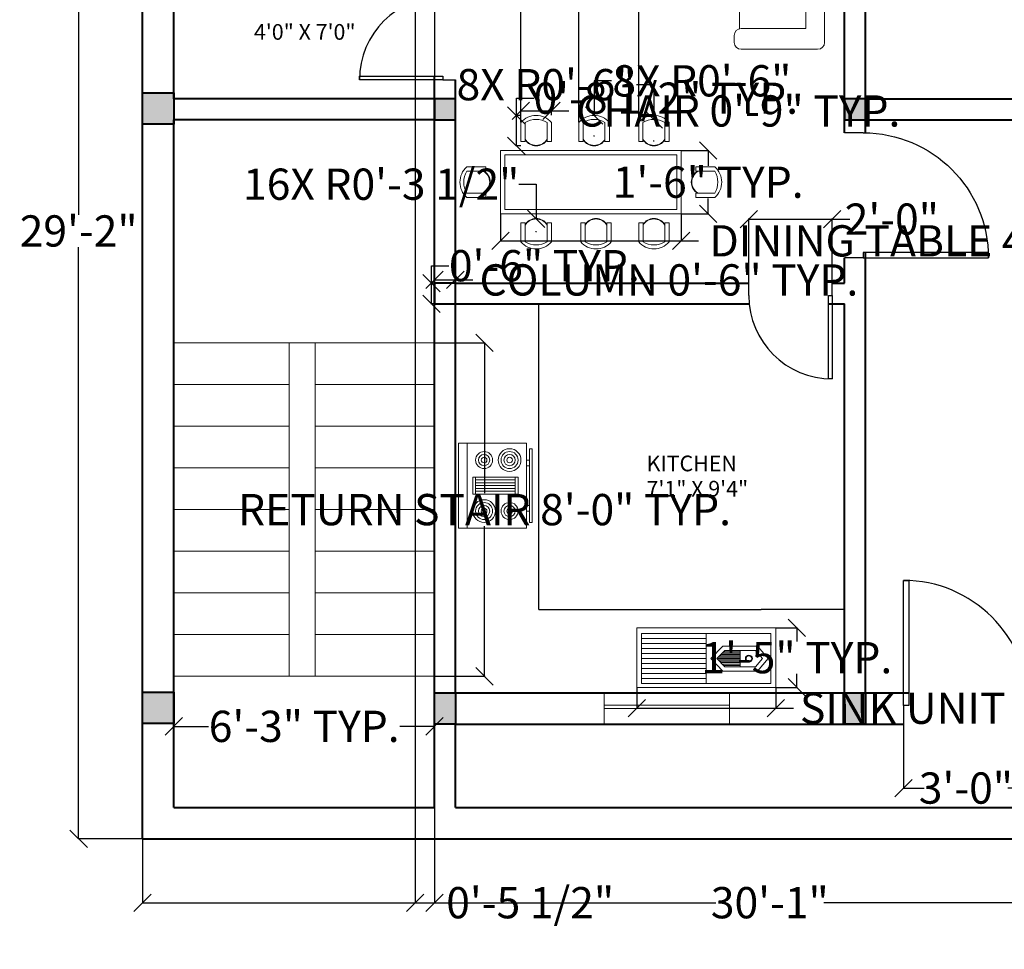
# Model space of a CAD drawing. Units: inches. Extents: x -19 to 1000, y -122 to 1144.
# Tile 1 of 8: x -14 to 270, y -122 to 146. Entities that reach past the tile are written whole.
import ezdxf

# ---------------------------------------------------------------- set-up
doc = ezdxf.new("R2010")
doc.units = ezdxf.units.IN
doc.header["$MEASUREMENT"] = 0
for name, color, linetype, lineweight in [('A-ANNO-DIMS', 191, 'Continuous', 18), ('A-AREA-IDEN', 1, 'Continuous', 18), ('A-COLS', 4, 'Continuous', 40), ('A-COLS-PATT', 220, 'Continuous', 13), ('A-EQPM', 120, 'Continuous', 18), ('A-FLOR-CASE', 254, 'Continuous', 25), ('A-FLOR-FIXT', 8, 'Continuous', 18), ('A-FLOR-STRS', 241, 'Continuous', 18), ('DOORS', 2, 'Continuous', 25), ('FURNITURE', 120, 'Continuous', 18), ('WALLS', 4, 'Continuous', 40), ('WINDOWS', 3, 'Continuous', 18)]:
    doc.layers.add(name, color=color, linetype=linetype, lineweight=lineweight)
doc.styles.get("Standard").update_dxf_attribs({"font": 'arial.ttf'})
doc.dimstyles.get("Standard").update_dxf_attribs({"dimtxt": 9, "dimasz": 5, "dimexe": 0.18, "dimexo": 0.0625, "dimgap": 0.09, "dimtad": 0, "dimtih": 1, "dimtoh": 1, "dimdec": 0, "dimzin": 0, "dimdsep": 46, "dimlunit": 3, "dimtxsty": 'Standard', "dimblk": 'OBLIQUE', "dimcen": 0.09, "dimadec": 0, "dimazin": 0, "dimtfac": 1, "dimtdec": 0, "dimtofl": 0, "dimtmove": 0, "dimatfit": 3, "dimfxl": 1, "dimtolj": 1, "dimtzin": 0, "dimarcsym": 0})

# ---------------------------------------------------------------- blocks, each defined once
blk = doc.blocks.new('Range-Oven - 30 in top')
for p, q in [((0, -3), (30, -3)), ((12, -6), (18, -6)), ((13, -20), (13, -6)), ((14, -6), (14, -20)), ((15, -20), (15, -6)), ((16, -6), (16, -20)), ((17, -20), (17, -6)), ((18, -20), (12, -20)), ((6, -24), (6, -25)), ((8, -25), (8, -24)), ((22, -25), (22, -24)), ((24, -24), (24, -25))]:
    blk.add_line(p, q)
for points in [[(0, -24), (0, 0), (30, 0), (30, -24)], [(12, -21), (12, -5), (18, -5), (18, -21)], [(2, -26), (2, -25), (28, -25), (28, -26)]]:
    blk.add_lwpolyline(points, close=True)
for centre, radius in [((6, -9), 4), ((6, -9), 3), ((24, -9), 3), ((6, -9), 2), ((6, -9), 1), ((24, -9), 2), ((24, -9), 1), ((6, -18), 3), ((6, -18), 2), ((6, -18), 1), ((24, -18), 4), ((24, -18), 3), ((24, -18), 2), ((24, -18), 1)]:
    blk.add_circle(centre, radius)
blk = doc.blocks.new('*U3')
for p, q in [((0, 0), (0, -6)), ((40, 0), (40, -6))]:
    blk.add_line(p, q)
blk.add_lwpolyline([(0, 0), (0, 40), (1.75, 40), (1.75, 0)], close=True)
blk.add_arc((0, 0), 40, 0, 90)
blk = doc.blocks.new('SOFA-THREE-SEAT')
for p, q in [((2, 84), (24, 84)), ((0, 78), (0, 82)), ((26, 82), (26, 2)), ((0, 78), (20.62, 78)), ((1.56, 78), (1.56, 56)), ((20.62, 78), (20.62, 6)), ((3.56, 54), (20.62, 54)), ((3.56, 54), (3.56, 54)), ((1.56, 52), (1.56, 32)), ((3.56, 30), (20.62, 30)), ((3.56, 30), (3.56, 30)), ((1.56, 28), (1.56, 6)), ((2, 6), (20.62, 6)), ((0, 2), (0, 4)), ((24, 0), (2, 0))]:
    blk.add_line(p, q)
for centre, start, end in [((2, 82), 90, 180), ((24, 82), 0, 90), ((3.56, 56), 180, 270), ((3.56, 52), 90, 180), ((3.56, 32), 180, 270), ((3.56, 28), 90, 180), ((2, 4), 90, 180), ((2, 2), 180, 270), ((24, 2), 270, 0)]:
    blk.add_arc(centre, 2, start, end)
blk = doc.blocks.new('TABLE-DINING')
for points in [[(51.97, 0), (0, 0), (0, 18.2), (51.97, 18.2)], [(50.72, 1.24), (1.24, 1.24), (1.24, 16.96), (50.72, 16.96)]]:
    blk.add_lwpolyline(points, close=True)
blk = doc.blocks.new('CHAIR-DINING')
for p, q in [((0, 1.28), (0, 6.78)), ((1.24, 1.28), (1.24, 6.78)), ((7.52, 1.28), (7.52, 6.78)), ((8.77, 1.28), (8.77, 6.78)), ((0, 1.28), (1.24, 1.28)), ((7.52, 1.28), (8.77, 1.28))]:
    blk.add_line(p, q)
for centre, radius, start, end in [((4.38, 2.88), 5.87, 41.6504, 138.3496), ((4.38, 1.47), 6.17, 59.4137, 120.5863), ((4.38, 3.81), 3.65, 210.7965, 329.2035), ((4.38, 3.65), 3.65, 210.7965, 329.2035)]:
    blk.add_arc(centre, radius, start, end)
blk = doc.blocks.new('SINK-WITH-DRAINBOARD')
for p, q in [((19.91, 15.5), (1.26, 15.5)), ((19.91, 1.08), (19.91, 15.5)), ((19.91, 14.06), (1.26, 14.06)), ((19.91, 12.62), (1.26, 12.62)), ((24.75, 11.88), (21.21, 8.28)), ((24.75, 11.88), (34.73, 11.88)), ((34.73, 11.88), (37.76, 8.28)), ((19.91, 11.17), (1.26, 11.17)), ((19.91, 9.73), (1.26, 9.73)), ((25.28, 10.62), (22.97, 8.28)), ((23.36, 8.67), (29.71, 8.67)), ((23.74, 9.06), (29.71, 9.06)), ((24.12, 9.45), (29.71, 9.45)), ((24.51, 9.84), (29.71, 9.84)), ((24.89, 10.23), (29.71, 10.23)), ((25.28, 10.62), (34.14, 10.62)), ((25.28, 10.62), (29.71, 10.62)), ((29.71, 5.94), (29.71, 10.62)), ((34.14, 10.62), (36.12, 8.28)), ((19.91, 8.29), (1.26, 8.29)), ((19.91, 6.85), (1.26, 6.85)), ((24.75, 4.68), (21.21, 8.28)), ((25.28, 5.94), (22.97, 8.28)), ((22.97, 8.28), (29.71, 8.28)), ((23.36, 7.89), (29.71, 7.89)), ((23.74, 7.5), (29.71, 7.5)), ((24.12, 7.11), (29.71, 7.11)), ((24.51, 6.72), (29.71, 6.72)), ((24.89, 6.33), (29.71, 6.33)), ((25.28, 5.94), (34.14, 5.94)), ((34.14, 5.94), (36.12, 8.28)), ((34.73, 4.68), (37.76, 8.28)), ((19.91, 5.4), (1.26, 5.4)), ((19.91, 3.96), (1.26, 3.96)), ((24.75, 4.68), (34.73, 4.68)), ((19.91, 2.52), (1.26, 2.52))]:
    blk.add_line(p, q)
for points in [[(40, 0), (0, 0), (0, 17.1), (40, 17.1)], [(38.55, 1.08), (1.26, 1.08), (1.26, 15.5), (38.55, 15.5)]]:
    blk.add_lwpolyline(points, close=True)
for radius in [1.01, 0.803]:
    blk.add_circle((32.21, 8.28), radius)
blk = doc.blocks.new('STAIR-RETURN-PLAN')
for p, q in [((75, 96), (0, 96)), ((33.21, 0), (33.21, 96)), ((40.68, 0), (40.68, 96)), ((33.21, 84), (0, 84)), ((75, 84), (40.68, 84)), ((33.21, 72), (0, 72)), ((75, 72), (40.68, 72)), ((33.21, 60), (0, 60)), ((75, 60), (40.68, 60)), ((33.21, 48), (0, 48)), ((75, 48), (40.68, 48)), ((33.21, 36), (0, 36)), ((75, 36), (40.68, 36)), ((33.21, 24), (0, 24)), ((75, 24), (40.68, 24)), ((33.21, 12), (0, 12)), ((75, 12), (40.68, 12)), ((75, 0), (0, 0))]:
    blk.add_line(p, q)
blk = doc.blocks.new('WIN-36-PLAN')
for p, q in [((0, 4.5), (0, 9)), ((0, 9), (0, 0)), ((36, 9), (36, 0)), ((0, 5.5), (36, 5.5)), ((0, 5.5), (36, 5.5)), ((0, 4.5), (36, 4.5))]:
    blk.add_line(p, q)
blk = doc.blocks.new('COLUMN-9X9')
blk.add_lwpolyline([(0, 9), (9, 9), (9, 0), (0, 0)], close=True)
blk = doc.blocks.new('COLUMN-6X6')
blk.add_lwpolyline([(6, 6), (0, 6), (0, 0), (6, 0)], close=True)
blk = doc.blocks.new('COLUMN-6X9')
blk.add_lwpolyline([(0, 9), (6, 9), (6, 0), (0, 0)], close=True)
blk = doc.blocks.new('_Oblique')
at = {"color": 0, "linetype": 'ByBlock', "lineweight": -2}
blk.add_line((-0.5, -0.5), (0.5, 0.5), dxfattribs=at)
blk = doc.blocks.new('*D35')
at = {"layer": 'A-ANNO-DIMS', "color": 0, "lineweight": -2, "transparency": 16777216}
for p, q in [((105.64, 69.78), (105.64, 70.79)), ((105.64, 70.61), (111.64, 70.61)), ((111.64, 69.78), (111.64, 70.79)), ((111.64, 70.61), (116.64, 70.61))]:
    blk.add_line(p, q, dxfattribs=at)
at = {"layer": 'Defpoints', "color": 0, "transparency": 16777216}
for p in [(105.64, 69.71), (111.64, 70.61), (111.64, 69.71)]:
    blk.add_point(p, dxfattribs=at)
at = {"layer": 'A-ANNO-DIMS', "color": 0, "lineweight": -2, "transparency": 16777216, "xscale": 5, "yscale": 5, "zscale": 5, "rotation": 180}
blk.add_blockref('_Oblique', (105.64, 70.61), dxfattribs=at)
at = {"layer": 'A-ANNO-DIMS', "color": 0, "lineweight": -2, "transparency": 16777216, "xscale": 5, "yscale": 5, "zscale": 5}
blk.add_blockref('_Oblique', (111.64, 70.61), dxfattribs=at)
at = {"layer": 'A-ANNO-DIMS', "color": 0, "transparency": 16777216, "insert": (173.1, 70.61), "char_height": 9, "attachment_point": 5}
blk.add_mtext('\\A1;COLUMN 0\'-6" TYP.', dxfattribs=at)
blk = doc.blocks.new('*D36')
at = {"layer": 'A-ANNO-DIMS', "color": 0, "lineweight": -2, "transparency": 16777216}
for p, q in [((104.74, 69.71), (104.74, 74.71)), ((104.74, 74.71), (109.74, 74.71)), ((105.58, 69.71), (104.56, 69.71)), ((104.74, 63.71), (104.74, 69.71)), ((105.58, 63.71), (104.56, 63.71))]:
    blk.add_line(p, q, dxfattribs=at)
at = {"layer": 'Defpoints', "color": 0, "transparency": 16777216}
for p in [(104.74, 69.71), (105.64, 69.71), (105.64, 63.71)]:
    blk.add_point(p, dxfattribs=at)
at = {"layer": 'A-ANNO-DIMS', "color": 0, "lineweight": -2, "transparency": 16777216, "xscale": 5, "yscale": 5, "zscale": 5}
for p, rotation in [((104.74, 69.71), 90), ((104.74, 63.71), 270)]:
    blk.add_blockref('_Oblique', p, dxfattribs=dict(at, rotation=rotation))
at = {"layer": 'A-ANNO-DIMS', "color": 0, "transparency": 16777216, "insert": (137.26, 74.71), "char_height": 9, "attachment_point": 5}
blk.add_mtext('\\A1;0\'-6" TYP.', dxfattribs=at)
blk = doc.blocks.new('*D39')
at = {"layer": 'A-ANNO-DIMS', "color": 0, "lineweight": -2, "transparency": 16777216}
for p, q in [((130.52, 118.01), (130.52, 119.44)), ((130.52, 119.26), (139.28, 119.26)), ((139.28, 118.01), (139.28, 119.44)), ((139.28, 119.26), (144.28, 119.26))]:
    blk.add_line(p, q, dxfattribs=at)
at = {"layer": 'Defpoints', "color": 0, "transparency": 16777216}
for p in [(139.28, 119.26), (130.52, 117.94), (139.28, 117.94)]:
    blk.add_point(p, dxfattribs=at)
at = {"layer": 'A-ANNO-DIMS', "color": 0, "lineweight": -2, "transparency": 16777216, "xscale": 5, "yscale": 5, "zscale": 5, "rotation": 180}
blk.add_blockref('_Oblique', (130.52, 119.26), dxfattribs=at)
at = {"layer": 'A-ANNO-DIMS', "color": 0, "lineweight": -2, "transparency": 16777216, "xscale": 5, "yscale": 5, "zscale": 5}
blk.add_blockref('_Oblique', (139.28, 119.26), dxfattribs=at)
at = {"layer": 'A-ANNO-DIMS', "color": 0, "transparency": 16777216, "insert": (193.06, 119.26), "char_height": 9, "attachment_point": 5}
blk.add_mtext('\\A1;CHAIR 0\'-9" TYP.', dxfattribs=at)
blk = doc.blocks.new('*D40')
at = {"layer": 'A-ANNO-DIMS', "color": 0, "lineweight": -2, "transparency": 16777216}
for p, q in [((129.2, 117.94), (129.2, 122.94)), ((129.2, 122.94), (134.2, 122.94)), ((130.46, 117.94), (129.02, 117.94)), ((129.2, 109.2), (129.2, 117.94)), ((130.46, 109.2), (129.02, 109.2))]:
    blk.add_line(p, q, dxfattribs=at)
at = {"layer": 'Defpoints', "color": 0, "transparency": 16777216}
for p in [(129.2, 117.94), (130.52, 117.94), (130.52, 109.2)]:
    blk.add_point(p, dxfattribs=at)
at = {"layer": 'A-ANNO-DIMS', "color": 0, "lineweight": -2, "transparency": 16777216, "xscale": 5, "yscale": 5, "zscale": 5}
for p, rotation in [((129.2, 117.94), 90), ((129.2, 109.2), 270)]:
    blk.add_blockref('_Oblique', p, dxfattribs=dict(at, rotation=rotation))
at = {"layer": 'A-ANNO-DIMS', "color": 0, "transparency": 16777216, "insert": (172.21, 122.94), "char_height": 9, "attachment_point": 5}
blk.add_mtext('\\A1;0\'-8 1/2" TYP.', dxfattribs=at)
blk = doc.blocks.new('*D59')
at = {"layer": 'A-ANNO-DIMS', "color": 0, "lineweight": -2, "transparency": 16777216}
for p, q in [((124.63, 89.6), (124.63, 81.68)), ((176.6, 89.6), (176.6, 81.68)), ((124.63, 81.86), (176.6, 81.86)), ((176.6, 81.86), (181.6, 81.86))]:
    blk.add_line(p, q, dxfattribs=at)
at = {"layer": 'Defpoints', "color": 0, "transparency": 16777216}
for p in [(124.63, 89.66), (176.6, 89.66), (176.6, 81.86)]:
    blk.add_point(p, dxfattribs=at)
at = {"layer": 'A-ANNO-DIMS', "color": 0, "lineweight": -2, "transparency": 16777216, "xscale": 5, "yscale": 5, "zscale": 5, "rotation": 180}
blk.add_blockref('_Oblique', (124.63, 81.86), dxfattribs=at)
at = {"layer": 'A-ANNO-DIMS', "color": 0, "lineweight": -2, "transparency": 16777216, "xscale": 5, "yscale": 5, "zscale": 5}
blk.add_blockref('_Oblique', (176.6, 81.86), dxfattribs=at)
at = {"layer": 'A-ANNO-DIMS', "color": 0, "transparency": 16777216, "insert": (254.31, 81.86), "char_height": 9, "attachment_point": 5}
blk.add_mtext('\\A1;DINING TABLE 4\'-4" TYP.', dxfattribs=at)
blk = doc.blocks.new('*D60')
at = {"layer": 'A-ANNO-DIMS', "color": 0, "lineweight": -2, "transparency": 16777216}
for p, q in [((176.66, 107.86), (184.58, 107.86)), ((184.4, 107.86), (184.4, 103.44)), ((184.4, 89.66), (184.4, 94.07)), ((176.66, 89.66), (184.58, 89.66))]:
    blk.add_line(p, q, dxfattribs=at)
at = {"layer": 'Defpoints', "color": 0, "transparency": 16777216}
for p in [(176.6, 107.86), (184.4, 107.86), (176.6, 89.66)]:
    blk.add_point(p, dxfattribs=at)
at = {"layer": 'A-ANNO-DIMS', "color": 0, "lineweight": -2, "transparency": 16777216, "xscale": 5, "yscale": 5, "zscale": 5}
for p, rotation in [((184.4, 107.86), 90), ((184.4, 89.66), 270)]:
    blk.add_blockref('_Oblique', p, dxfattribs=dict(at, rotation=rotation))
at = {"layer": 'A-ANNO-DIMS', "color": 0, "transparency": 16777216, "insert": (184.4, 98.76), "char_height": 9, "attachment_point": 5}
blk.add_mtext('\\A1;1\'-6" TYP.', dxfattribs=at)
blk = doc.blocks.new('*D63')
at = {"layer": 'A-ANNO-DIMS', "color": 0, "lineweight": -2, "transparency": 16777216}
for p, q in [((163.91, -46.76), (163.91, -52.87)), ((203.91, -46.76), (203.91, -52.87)), ((163.91, -52.69), (203.91, -52.69)), ((203.91, -52.69), (208.91, -52.69))]:
    blk.add_line(p, q, dxfattribs=at)
at = {"layer": 'Defpoints', "color": 0, "transparency": 16777216}
for p in [(163.91, -46.69), (203.91, -46.69), (203.91, -52.69)]:
    blk.add_point(p, dxfattribs=at)
at = {"layer": 'A-ANNO-DIMS', "color": 0, "lineweight": -2, "transparency": 16777216, "xscale": 5, "yscale": 5, "zscale": 5, "rotation": 180}
blk.add_blockref('_Oblique', (163.91, -52.69), dxfattribs=at)
at = {"layer": 'A-ANNO-DIMS', "color": 0, "lineweight": -2, "transparency": 16777216, "xscale": 5, "yscale": 5, "zscale": 5}
blk.add_blockref('_Oblique', (203.91, -52.69), dxfattribs=at)
at = {"layer": 'A-ANNO-DIMS', "color": 0, "transparency": 16777216, "insert": (269.24, -52.69), "char_height": 9, "attachment_point": 5}
blk.add_mtext('\\A1;SINK UNIT 3\'-4" TYP.', dxfattribs=at)
blk = doc.blocks.new('*D64')
at = {"layer": 'A-ANNO-DIMS', "color": 0, "lineweight": -2, "transparency": 16777216}
for p, q in [((203.98, -29.6), (210.09, -29.6)), ((209.91, -29.6), (209.91, -33.46)), ((209.91, -46.69), (209.91, -42.83)), ((203.98, -46.69), (210.09, -46.69))]:
    blk.add_line(p, q, dxfattribs=at)
at = {"layer": 'Defpoints', "color": 0, "transparency": 16777216}
for p in [(203.91, -29.6), (209.91, -29.6), (203.91, -46.69)]:
    blk.add_point(p, dxfattribs=at)
at = {"layer": 'A-ANNO-DIMS', "color": 0, "lineweight": -2, "transparency": 16777216, "xscale": 5, "yscale": 5, "zscale": 5}
for p, rotation in [((209.91, -29.6), 90), ((209.91, -46.69), 270)]:
    blk.add_blockref('_Oblique', p, dxfattribs=dict(at, rotation=rotation))
at = {"layer": 'A-ANNO-DIMS', "color": 0, "transparency": 16777216, "insert": (209.91, -38.14), "char_height": 9, "attachment_point": 5}
blk.add_mtext('\\A1;1\'-5" TYP.', dxfattribs=at)
blk = doc.blocks.new('*D69')
at = {"layer": 'A-ANNO-DIMS', "color": 0, "lineweight": -2, "transparency": 16777216}
for p, q in [((105.7, 52.48), (120.22, 52.48)), ((120.04, 52.48), (120.04, 9.22)), ((120.04, -43.52), (120.04, -0.26)), ((105.7, -43.52), (120.22, -43.52))]:
    blk.add_line(p, q, dxfattribs=at)
at = {"layer": 'Defpoints', "color": 0, "transparency": 16777216}
for p in [(105.64, 52.48), (120.04, 52.48), (105.64, -43.52)]:
    blk.add_point(p, dxfattribs=at)
at = {"layer": 'A-ANNO-DIMS', "color": 0, "lineweight": -2, "transparency": 16777216, "xscale": 5, "yscale": 5, "zscale": 5}
for p, rotation in [((120.04, 52.48), 90), ((120.04, -43.52), 270)]:
    blk.add_blockref('_Oblique', p, dxfattribs=dict(at, rotation=rotation))
at = {"layer": 'A-ANNO-DIMS', "color": 0, "transparency": 16777216, "insert": (120.04, 4.48), "char_height": 9, "attachment_point": 5}
blk.add_mtext('\\A1;RETURN STAIR 8\'-0" TYP.', dxfattribs=at)
blk = doc.blocks.new('*D70')
at = {"layer": 'A-ANNO-DIMS', "color": 0, "lineweight": -2, "transparency": 16777216}
for p, q in [((30.64, -43.58), (30.64, -58.1)), ((105.64, -43.58), (105.64, -58.1)), ((30.64, -57.92), (40.6, -57.92)), ((105.64, -57.92), (95.69, -57.92))]:
    blk.add_line(p, q, dxfattribs=at)
at = {"layer": 'Defpoints', "color": 0, "transparency": 16777216}
for p in [(30.64, -43.52), (105.64, -43.52), (105.64, -57.92)]:
    blk.add_point(p, dxfattribs=at)
at = {"layer": 'A-ANNO-DIMS', "color": 0, "lineweight": -2, "transparency": 16777216, "xscale": 5, "yscale": 5, "zscale": 5, "rotation": 180}
blk.add_blockref('_Oblique', (30.64, -57.92), dxfattribs=at)
at = {"layer": 'A-ANNO-DIMS', "color": 0, "lineweight": -2, "transparency": 16777216, "xscale": 5, "yscale": 5, "zscale": 5}
blk.add_blockref('_Oblique', (105.64, -57.92), dxfattribs=at)
at = {"layer": 'A-ANNO-DIMS', "color": 0, "transparency": 16777216, "insert": (68.14, -57.92), "char_height": 9, "attachment_point": 5}
blk.add_mtext('\\A1;6\'-3" TYP.', dxfattribs=at)
blk = doc.blocks.new('*D83')
at = {"layer": 'A-ANNO-DIMS', "color": 0, "lineweight": -2, "transparency": 16777216}
for p, q in [((21.64, -90.36), (21.64, -108.87)), ((382.64, -90.36), (382.64, -108.87)), ((21.64, -108.69), (186.6, -108.69)), ((382.64, -108.69), (217.69, -108.69))]:
    blk.add_line(p, q, dxfattribs=at)
at = {"layer": 'Defpoints', "color": 0, "transparency": 16777216}
for p in [(21.64, -90.29), (382.64, -90.29), (382.64, -108.69)]:
    blk.add_point(p, dxfattribs=at)
at = {"layer": 'A-ANNO-DIMS', "color": 0, "lineweight": -2, "transparency": 16777216, "xscale": 5, "yscale": 5, "zscale": 5, "rotation": 180}
blk.add_blockref('_Oblique', (21.64, -108.69), dxfattribs=at)
at = {"layer": 'A-ANNO-DIMS', "color": 0, "lineweight": -2, "transparency": 16777216, "xscale": 5, "yscale": 5, "zscale": 5}
blk.add_blockref('_Oblique', (382.64, -108.69), dxfattribs=at)
at = {"layer": 'A-ANNO-DIMS', "color": 0, "transparency": 16777216, "insert": (202.14, -108.69), "char_height": 9, "attachment_point": 5}
blk.add_mtext('\\A1;30\'-1"', dxfattribs=at)
blk = doc.blocks.new('*D84')
at = {"layer": 'A-ANNO-DIMS', "color": 0, "lineweight": -2, "transparency": 16777216}
for p, q in [((21.58, 259.71), (3.06, 259.71)), ((3.24, 259.71), (3.24, 89.39)), ((3.24, -90.29), (3.24, 80.02)), ((21.58, -90.29), (3.06, -90.29))]:
    blk.add_line(p, q, dxfattribs=at)
at = {"layer": 'Defpoints', "color": 0, "transparency": 16777216}
for p in [(3.24, 259.71), (21.64, 259.71), (21.64, -90.29)]:
    blk.add_point(p, dxfattribs=at)
at = {"layer": 'A-ANNO-DIMS', "color": 0, "lineweight": -2, "transparency": 16777216, "xscale": 5, "yscale": 5, "zscale": 5}
for p, rotation in [((3.24, 259.71), 90), ((3.24, -90.29), 270)]:
    blk.add_blockref('_Oblique', p, dxfattribs=dict(at, rotation=rotation))
at = {"layer": 'A-ANNO-DIMS', "color": 0, "transparency": 16777216, "insert": (3.24, 84.71), "char_height": 9, "attachment_point": 5}
blk.add_mtext('\\A1;29\'-2"', dxfattribs=at)
blk = doc.blocks.new('*D94')
at = {"layer": 'A-ANNO-DIMS', "color": 0, "lineweight": -2, "transparency": 16777216}
for p, q in [((240.57, -57.36), (240.57, -75.87)), ((276.57, -57.36), (276.57, -75.87)), ((240.57, -75.69), (246.52, -75.69)), ((276.57, -75.69), (270.62, -75.69))]:
    blk.add_line(p, q, dxfattribs=at)
at = {"layer": 'Defpoints', "color": 0, "transparency": 16777216}
for p in [(240.57, -57.29), (276.57, -57.29), (240.57, -75.69)]:
    blk.add_point(p, dxfattribs=at)
at = {"layer": 'A-ANNO-DIMS', "color": 0, "lineweight": -2, "transparency": 16777216, "xscale": 5, "yscale": 5, "zscale": 5, "rotation": 180}
blk.add_blockref('_Oblique', (240.57, -75.69), dxfattribs=at)
at = {"layer": 'A-ANNO-DIMS', "color": 0, "lineweight": -2, "transparency": 16777216, "xscale": 5, "yscale": 5, "zscale": 5}
blk.add_blockref('_Oblique', (276.57, -75.69), dxfattribs=at)
at = {"layer": 'A-ANNO-DIMS', "color": 0, "transparency": 16777216, "insert": (258.57, -75.69), "char_height": 9, "attachment_point": 5}
blk.add_mtext('\\A1;3\'-0"', dxfattribs=at)
blk = doc.blocks.new('*D96')
at = {"layer": 'A-ANNO-DIMS', "color": 0, "lineweight": -2, "transparency": 16777216}
for p, q in [((196.12, 69.77), (196.12, 88.29)), ((196.12, 88.11), (220.12, 88.11)), ((220.12, 69.77), (220.12, 88.29)), ((220.12, 88.11), (225.12, 88.11))]:
    blk.add_line(p, q, dxfattribs=at)
at = {"layer": 'Defpoints', "color": 0, "transparency": 16777216}
for p in [(220.12, 88.11), (196.12, 69.71), (220.12, 69.71)]:
    blk.add_point(p, dxfattribs=at)
at = {"layer": 'A-ANNO-DIMS', "color": 0, "lineweight": -2, "transparency": 16777216, "xscale": 5, "yscale": 5, "zscale": 5, "rotation": 180}
blk.add_blockref('_Oblique', (196.12, 88.11), dxfattribs=at)
at = {"layer": 'A-ANNO-DIMS', "color": 0, "lineweight": -2, "transparency": 16777216, "xscale": 5, "yscale": 5, "zscale": 5}
blk.add_blockref('_Oblique', (220.12, 88.11), dxfattribs=at)
at = {"layer": 'A-ANNO-DIMS', "color": 0, "transparency": 16777216, "insert": (237.25, 88.11), "char_height": 9, "attachment_point": 5}
blk.add_mtext('\\A1;2\'-0"', dxfattribs=at)
blk = doc.blocks.new('*D100')
at = {"layer": 'A-ANNO-DIMS', "color": 0, "lineweight": -2, "transparency": 16777216}
for p, q in [((100.07, 171.74), (100.07, -108.87)), ((105.64, 166.64), (105.64, -108.87)), ((100.07, -108.69), (105.64, -108.69)), ((105.64, -108.69), (110.64, -108.69))]:
    blk.add_line(p, q, dxfattribs=at)
at = {"layer": 'Defpoints', "color": 0, "transparency": 16777216}
for p in [(100.07, 171.8), (105.64, 166.71), (105.64, -108.69)]:
    blk.add_point(p, dxfattribs=at)
at = {"layer": 'A-ANNO-DIMS', "color": 0, "lineweight": -2, "transparency": 16777216, "xscale": 5, "yscale": 5, "zscale": 5, "rotation": 180}
blk.add_blockref('_Oblique', (100.07, -108.69), dxfattribs=at)
at = {"layer": 'A-ANNO-DIMS', "color": 0, "lineweight": -2, "transparency": 16777216, "xscale": 5, "yscale": 5, "zscale": 5}
blk.add_blockref('_Oblique', (105.64, -108.69), dxfattribs=at)
at = {"layer": 'A-ANNO-DIMS', "color": 0, "transparency": 16777216, "insert": (133.18, -108.69), "char_height": 9, "attachment_point": 5}
blk.add_mtext('\\A1;0\'-5 1/2"', dxfattribs=at)
blk = doc.blocks.new('*D101')
at = {"layer": 'A-ANNO-DIMS', "color": 0, "lineweight": -2, "transparency": 16777216}
for p, q in [((130.52, 116.04), (130.52, 278.29)), ((130.52, 278.11), (147.19, 278.11)), ((147.19, 116.04), (147.19, 278.29)), ((147.19, 278.11), (152.19, 278.11))]:
    blk.add_line(p, q, dxfattribs=at)
at = {"layer": 'Defpoints', "color": 0, "transparency": 16777216}
for p in [(147.19, 278.11), (130.52, 115.98), (147.19, 115.98)]:
    blk.add_point(p, dxfattribs=at)
at = {"layer": 'A-ANNO-DIMS', "color": 0, "lineweight": -2, "transparency": 16777216, "xscale": 5, "yscale": 5, "zscale": 5, "rotation": 180}
blk.add_blockref('_Oblique', (130.52, 278.11), dxfattribs=at)
at = {"layer": 'A-ANNO-DIMS', "color": 0, "lineweight": -2, "transparency": 16777216, "xscale": 5, "yscale": 5, "zscale": 5}
blk.add_blockref('_Oblique', (147.19, 278.11), dxfattribs=at)
at = {"layer": 'A-ANNO-DIMS', "color": 0, "transparency": 16777216, "insert": (174.3, 278.11), "char_height": 9, "attachment_point": 5}
blk.add_mtext('\\A1;1\'-4 1/2"', dxfattribs=at)
blk = doc.blocks.new('*D102')
at = {"layer": 'A-ANNO-DIMS', "color": 0, "lineweight": -2, "transparency": 16777216}
for p, q in [((147.19, 116.04), (147.19, 278.29)), ((147.19, 278.11), (164.4, 278.11)), ((164.4, 116.04), (164.4, 278.29)), ((164.4, 278.11), (169.4, 278.11))]:
    blk.add_line(p, q, dxfattribs=at)
at = {"layer": 'Defpoints', "color": 0, "transparency": 16777216}
for p in [(164.4, 278.11), (147.19, 115.98), (164.4, 115.98)]:
    blk.add_point(p, dxfattribs=at)
at = {"layer": 'A-ANNO-DIMS', "color": 0, "lineweight": -2, "transparency": 16777216, "xscale": 5, "yscale": 5, "zscale": 5, "rotation": 180}
blk.add_blockref('_Oblique', (147.19, 278.11), dxfattribs=at)
at = {"layer": 'A-ANNO-DIMS', "color": 0, "lineweight": -2, "transparency": 16777216, "xscale": 5, "yscale": 5, "zscale": 5}
blk.add_blockref('_Oblique', (164.4, 278.11), dxfattribs=at)
at = {"layer": 'A-ANNO-DIMS', "color": 0, "transparency": 16777216, "insert": (181.03, 278.11), "char_height": 9, "attachment_point": 5}
blk.add_mtext('\\A1;1\'-5"', dxfattribs=at)
blk = doc.blocks.new('*D145')
at = {"layer": 'A-ANNO-DIMS', "color": 0, "lineweight": -2, "transparency": 16777216}
for p, q in [((163.79, 126.83), (168.79, 126.83)), ((168.79, 126.83), (168.79, 116.83)), ((168.7, 110.67), (168.88, 110.67)), ((168.79, 110.58), (168.79, 110.76))]:
    blk.add_line(p, q, dxfattribs=at)
at = {"layer": 'Defpoints', "color": 0, "transparency": 16777216}
for p in [(168.79, 116.83), (168.79, 110.67)]:
    blk.add_point(p, dxfattribs=at)
at = {"layer": 'A-ANNO-DIMS', "color": 0, "lineweight": -2, "transparency": 16777216, "xscale": 5, "yscale": 5, "zscale": 5, "rotation": 270.0019411470775}
blk.add_blockref('_Oblique', (168.79, 116.83), dxfattribs=at)
at = {"layer": 'A-ANNO-DIMS', "color": 0, "transparency": 16777216, "insert": (137.75, 126.83), "char_height": 9, "attachment_point": 5}
blk.add_mtext('\\A1;8X R0\'-6"', dxfattribs=at)
blk = doc.blocks.new('*D146')
at = {"layer": 'A-ANNO-DIMS', "color": 0, "lineweight": -2, "transparency": 16777216}
for p, q in [((156.57, 127.94), (151.57, 127.94)), ((151.57, 127.94), (151.57, 117.94)), ((151.48, 112.08), (151.66, 112.08)), ((151.57, 111.99), (151.57, 112.17))]:
    blk.add_line(p, q, dxfattribs=at)
at = {"layer": 'Defpoints', "color": 0, "transparency": 16777216}
for p in [(151.57, 117.94), (151.57, 112.08)]:
    blk.add_point(p, dxfattribs=at)
at = {"layer": 'A-ANNO-DIMS', "color": 0, "lineweight": -2, "transparency": 16777216, "xscale": 5, "yscale": 5, "zscale": 5, "rotation": 269.9952918261828}
blk.add_blockref('_Oblique', (151.57, 117.94), dxfattribs=at)
at = {"layer": 'A-ANNO-DIMS', "color": 0, "transparency": 16777216, "insert": (182.6, 127.94), "char_height": 9, "attachment_point": 5}
blk.add_mtext('\\A1;8X R0\'-6"', dxfattribs=at)
blk = doc.blocks.new('*D147')
at = {"layer": 'A-ANNO-DIMS', "color": 0, "lineweight": -2, "transparency": 16777216}
for p, q in [((129.9, 98.17), (134.9, 98.17)), ((134.9, 98.17), (134.9, 88.17)), ((134.81, 84.51), (134.99, 84.51)), ((134.9, 84.42), (134.9, 84.6))]:
    blk.add_line(p, q, dxfattribs=at)
at = {"layer": 'Defpoints', "color": 0, "transparency": 16777216}
for p in [(134.9, 88.17), (134.9, 84.51)]:
    blk.add_point(p, dxfattribs=at)
at = {"layer": 'A-ANNO-DIMS', "color": 0, "lineweight": -2, "transparency": 16777216, "xscale": 5, "yscale": 5, "zscale": 5, "rotation": 270.0077611997318}
blk.add_blockref('_Oblique', (134.9, 88.17), dxfattribs=at)
at = {"layer": 'A-ANNO-DIMS', "color": 0, "transparency": 16777216, "insert": (90.31, 98.17), "char_height": 9, "attachment_point": 5}
blk.add_mtext('\\A1;16X R0\'-3 1/2"', dxfattribs=at)

msp = doc.modelspace()

# ---------------------------------------------------------------- hatches: boundary and pattern name
at = {"layer": 'A-COLS-PATT'}
h = msp.add_hatch(color=256, dxfattribs=at)
h.dxf.hatch_style = 1
h.paths.add_polyline_path([(30.64, 259.71), (21.64, 259.71), (21.64, 250.71), (30.64, 250.71)])
h.paths.add_polyline_path([(113.34, 259.71), (104.34, 259.71), (104.34, 250.71), (113.34, 250.71)])
h.paths.add_polyline_path([(231.33, 259.71), (222.33, 259.71), (222.33, 250.71), (223.64, 250.71), (231.33, 250.71)])
h.paths.add_polyline_path([(382.64, 259.71), (373.64, 259.71), (373.64, 250.71), (382.64, 250.71)])
h.paths.add_polyline_path([(382.64, 124.35), (373.64, 124.35), (373.64, 115.35), (382.64, 115.35)])
h.paths.add_polyline_path([(382.64, -48.29), (373.64, -48.29), (373.64, -57.29), (382.64, -57.29)])
h.paths.add_polyline_path([(111.64, -48.29), (105.64, -48.29), (105.64, -57.29), (111.64, -57.29)])
h.paths.add_polyline_path([(30.64, -48.11), (21.64, -48.11), (21.64, -57.11), (30.64, -57.11)])
h.paths.add_polyline_path([(30.64, 124.5), (21.64, 124.5), (21.64, 115.5), (30.64, 115.5)])
h.paths.add_polyline_path([(111.64, 122.71), (105.64, 122.71), (105.64, 116.71), (111.64, 116.71)])
h.paths.add_polyline_path([(229.64, 122.71), (223.64, 122.71), (223.64, 116.71), (229.64, 116.71)])
h.paths.add_polyline_path([(229.64, -48.29), (223.64, -48.29), (223.64, -57.29), (229.64, -57.29)])

# ---------------------------------------------------------------- linework, layer by layer
at = {"layer": 'A-FLOR-CASE'}
for p, q in [((135.64, -24.29), (135.64, 63.71)), ((135.64, -24.29), (199.64, -24.29)), ((223.64, -24.29), (199.64, -24.29))]:
    msp.add_line(p, q, dxfattribs=at)
at = {"layer": 'WALLS'}
for p, q in [((21.64, -90.29), (21.64, 259.71)), ((223.64, 112.97), (223.64, 250.71)), ((229.64, 122.71), (229.64, 250.71)), ((30.64, 122.71), (30.64, 160.71)), ((105.64, -81.29), (105.64, 129.26)), ((111.64, 69.71), (111.64, 128.21)), ((105.64, 122.71), (30.64, 122.71)), ((229.64, 122.71), (373.64, 122.71)), ((30.64, -81.29), (30.64, 116.71)), ((105.64, 116.71), (30.64, 116.71)), ((229.64, 116.71), (373.64, 116.71)), ((229.64, 112.97), (229.64, 116.71)), ((223.64, 69.71), (223.64, 76.97)), ((229.64, -48.29), (229.64, 78.55)), ((111.64, 69.71), (196.12, 69.71)), ((220.12, 69.71), (223.64, 69.71)), ((111.64, 63.71), (196.24, 63.71)), ((111.64, -48.29), (111.64, 63.71)), ((219.07, 63.71), (223.64, 63.71)), ((223.64, -48.29), (223.64, 63.71)), ((111.64, -48.29), (223.64, -48.29)), ((229.64, -48.29), (242.15, -48.29)), ((111.64, -81.29), (111.64, -57.29)), ((111.64, -57.29), (223.64, -57.29)), ((223.64, -57.29), (240.57, -57.29)), ((30.64, -81.29), (105.64, -81.29)), ((111.64, -81.29), (223.64, -81.29)), ((223.64, -81.29), (373.64, -81.29)), ((21.64, -90.29), (223.64, -90.29)), ((223.64, -90.29), (382.64, -90.29))]:
    msp.add_line(p, q, dxfattribs=at)
msp.add_lwpolyline([(229.64, 63.71), (229.64, 63.71), (229.64, 69.71)], dxfattribs=at)

# ---------------------------------------------------------------- block references
at = {"layer": 'A-COLS'}
for name, p in [('COLUMN-9X9', (21.64, 115.5)), ('COLUMN-6X6', (105.64, 116.7)), ('COLUMN-6X6', (223.64, 116.7)), ('COLUMN-6X6', (105.64, 63.71)), ('COLUMN-9X9', (21.64, -57.11)), ('COLUMN-6X9', (105.64, -57.3)), ('COLUMN-6X9', (223.64, -57.3))]:
    msp.add_blockref(name, p, dxfattribs=at)
at = {"layer": 'A-EQPM', "xscale": 0.8155908971350484, "yscale": 0.8155908971350484, "zscale": 0.8155908971350484, "rotation": 90}
msp.add_blockref('Range-Oven - 30 in top', (112.58, -0.82), dxfattribs=at)
at = {"layer": 'A-FLOR-FIXT'}
msp.add_blockref('SINK-WITH-DRAINBOARD', (163.91, -46.69), dxfattribs=at)
at = {"layer": 'A-FLOR-STRS'}
msp.add_blockref('STAIR-RETURN-PLAN', (30.64, -43.52), dxfattribs=at)
at = {"layer": 'DOORS'}
for p, xscale, yscale, zscale, rotation in [((108.04, 128.21), 0.6, 0.6, 0.6, 90), ((229.04, 76.97), -0.9, 0.9, 0.9, 270), ((220.12, 66.11), 0.6, 0.6, 0.6, 180)]:
    msp.add_blockref('*U3', p, dxfattribs=dict(at, xscale=xscale, yscale=yscale, zscale=zscale, rotation=rotation))
at = {"layer": 'DOORS', "xscale": 0.9, "yscale": 0.9, "zscale": 0.9}
msp.add_blockref('*U3', (240.57, -51.89), dxfattribs=at)
at = {"layer": 'FURNITURE'}
for name, p in [('SOFA-THREE-SEAT', (191.9, 137.01)), ('CHAIR-DINING', (130.52, 109.2)), ('CHAIR-DINING', (147.19, 109.2)), ('CHAIR-DINING', (164.4, 109.2)), ('TABLE-DINING', (124.63, 89.66))]:
    msp.add_blockref(name, p, dxfattribs=at)
for p, rotation in [((121.7, 94.37), 89.99999999999969), ((179.54, 103.14), 269.9999999999991), ((139.28, 88.32), 180), ((156.5, 88.32), 180), ((173.17, 88.32), 180)]:
    msp.add_blockref('CHAIR-DINING', p, dxfattribs=dict(at, rotation=rotation))
at = {"layer": 'WINDOWS'}
msp.add_blockref('WIN-36-PLAN', (154.51, -57.3), dxfattribs=at)

# ---------------------------------------------------------------- texts
at = {"layer": 'A-AREA-IDEN'}
for s, height, p in [('4\'0" X 7\'0"', 4.5155, (53.69, 139.75)), ('KITCHEN', 4.516, (166.68, 15.51)), ('7\'1" X 9\'4"', 4.5155, (166.68, 8.25))]:
    msp.add_text(s, height=height, dxfattribs=at).set_placement(p)

# ---------------------------------------------------------------- dimensions: what is measured, and where the dimension line sits
at = {"layer": 'A-ANNO-DIMS'}
for base, p1, p2, picture, middle in [((147.19, 278.11), (130.52, 115.98), (147.19, 115.98), '*D101', (174.3, 278.11)), ((164.4, 278.11), (147.19, 115.98), (164.4, 115.98), '*D102', (181.03, 278.11)), ((105.64, -108.69), (100.07, 171.8), (105.64, 166.71), '*D100', (133.18, -108.69)), ((220.12, 88.11), (196.12, 69.71), (220.12, 69.71), '*D96', (237.25, 88.11)), ((382.64, -108.69), (21.64, -90.29), (382.64, -90.29), '*D83', (202.14, -108.69))]:
    dim = msp.add_linear_dim(base=base, p1=p1, p2=p2, dimstyle='Standard', override={"dimdec": 1, "dimlfac": 1, "dimrnd": 0, "dimzin": 1, "dimdsep": 46, "dimlunit": 4, "dimfrac": 2}, dxfattribs=at)
    dim.commit()
    dim.dimension.update_dxf_attribs({"geometry": picture, "text_midpoint": middle})
for base, p1, p2, angle, picture, middle in [((3.24, 259.71), (21.64, -90.29), (21.64, 259.71), 90, '*D84', (3.24, 84.71)), ((240.57, -75.69), (276.57, -57.29), (240.57, -57.29), 180, '*D94', (258.57, -75.69))]:
    dim = msp.add_linear_dim(base=base, p1=p1, p2=p2, angle=angle, dimstyle='Standard', override={"dimdec": 1, "dimlfac": 1, "dimrnd": 0, "dimzin": 1, "dimdsep": 46, "dimlunit": 4, "dimfrac": 2}, dxfattribs=at)
    dim.commit()
    dim.dimension.update_dxf_attribs({"geometry": picture, "text_midpoint": middle})
for base, p1, p2, text, picture, middle in [((129.2, 117.94), (130.52, 109.2), (130.52, 117.94), '<> TYP.', '*D40', (172.21, 122.94)), ((184.4, 107.86), (176.6, 89.66), (176.6, 107.86), '<> TYP.', '*D60', (184.4, 98.76)), ((104.74, 69.71), (105.64, 63.71), (105.64, 69.71), '<> TYP.', '*D36', (137.26, 74.71)), ((120.04, 52.48), (105.64, -43.52), (105.64, 52.48), 'RETURN STAIR <> TYP.', '*D69', (120.04, 4.48)), ((209.91, -29.6), (203.91, -46.69), (203.91, -29.6), '<> TYP.', '*D64', (209.91, -38.14))]:
    dim = msp.add_linear_dim(base=base, p1=p1, p2=p2, angle=90, text=text, dimstyle='Standard', override={"dimdec": 1, "dimlfac": 1, "dimrnd": 0, "dimzin": 1, "dimdsep": 46, "dimlunit": 4, "dimfrac": 2}, dxfattribs=at)
    dim.commit()
    dim.dimension.update_dxf_attribs({"geometry": picture, "text_midpoint": middle})
for center, mpoint, text, picture, middle in [((168.79, 110.67), (168.79, 116.83), '8X <>', '*D145', (137.75, 126.83)), ((151.57, 112.08), (151.57, 117.94), '8X <>', '*D146', (182.6, 127.94)), ((134.9, 84.51), (134.9, 88.17), '16X <>', '*D147', (90.31, 98.17))]:
    dim = msp.add_radius_dim(center=center, mpoint=mpoint, text=text, dimstyle='Standard', override={"dimdec": 1, "dimlfac": 1, "dimrnd": 0, "dimzin": 1, "dimdsep": 46, "dimlunit": 4, "dimfrac": 2}, dxfattribs=at)
    dim.commit()
    dim.dimension.update_dxf_attribs({"geometry": picture, "text_midpoint": middle})
for base, p1, p2, text, picture, middle in [((139.28, 119.26), (130.52, 117.94), (139.28, 117.94), 'CHAIR <> TYP.', '*D39', (193.06, 119.26)), ((176.6, 81.86), (124.63, 89.66), (176.6, 89.66), 'DINING TABLE <> TYP.', '*D59', (254.31, 81.86)), ((111.64, 70.61), (105.64, 69.71), (111.64, 69.71), 'COLUMN <> TYP.', '*D35', (173.1, 70.61)), ((203.91, -52.69), (163.91, -46.69), (203.91, -46.69), 'SINK UNIT <> TYP.', '*D63', (269.24, -52.69)), ((105.64, -57.92), (30.64, -43.52), (105.64, -43.52), '<> TYP.', '*D70', (68.14, -57.92))]:
    dim = msp.add_linear_dim(base=base, p1=p1, p2=p2, text=text, dimstyle='Standard', override={"dimdec": 1, "dimlfac": 1, "dimrnd": 0, "dimzin": 1, "dimdsep": 46, "dimlunit": 4, "dimfrac": 2}, dxfattribs=at)
    dim.commit()
    dim.dimension.update_dxf_attribs({"geometry": picture, "text_midpoint": middle})

doc.saveas('drawing.dxf')
